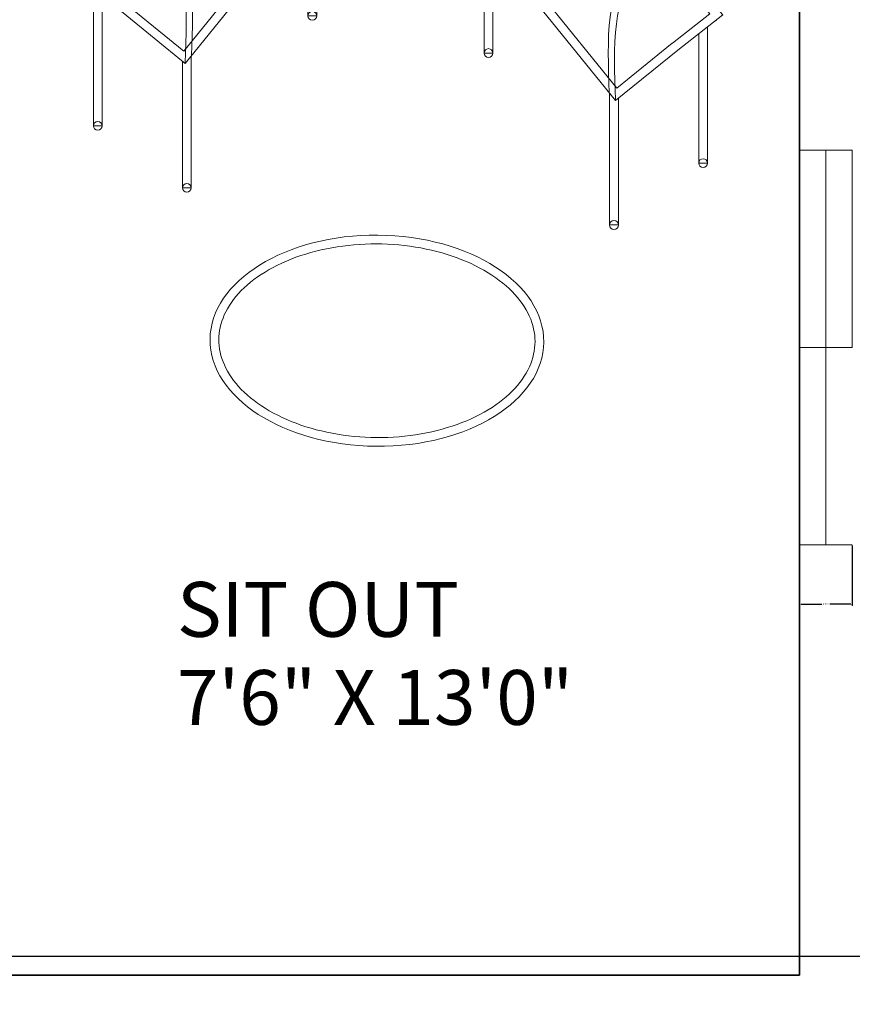
# Model space of a CAD drawing. Units: inches. Extents: x -61 to 1599, y -1316 to 257.
# Tile 192 of 204: x 1003 to 1098, y -173 to -61. Entities that reach past the tile are written whole.
import ezdxf

# ---------------------------------------------------------------- set-up
doc = ezdxf.new("R2010")
doc.units = ezdxf.units.IN
doc.header["$MEASUREMENT"] = 0
for name, color, linetype, lineweight in [('A-ANNO-DIMS', 2, 'Continuous', 18), ('A-AREA-IDEN', 1, 'Continuous', 18), ('FURNITURE', 83, 'Continuous', 18), ('WALLS', 4, 'Continuous', 35), ('WINDOWS', 220, 'Continuous', 18)]:
    doc.layers.add(name, color=color, linetype=linetype, lineweight=lineweight)
doc.styles.get("Standard").update_dxf_attribs({"font": 'arial.ttf'})
doc.dimstyles.get("Standard").update_dxf_attribs({"dimtxt": 0.18, "dimasz": 0.18, "dimexe": 0.18, "dimexo": 0.0625, "dimgap": 0.09, "dimtad": 0, "dimtih": 1, "dimtoh": 1, "dimdec": 0, "dimzin": 0, "dimdsep": 46, "dimlunit": 3, "dimtxsty": 'Standard', "dimcen": 0.09, "dimadec": 0, "dimazin": 0, "dimtfac": 1, "dimtdec": 0, "dimtofl": 0, "dimtmove": 0, "dimatfit": 3, "dimfxl": 1, "dimtolj": 1, "dimtzin": 0, "dimarcsym": 0})

# ---------------------------------------------------------------- blocks, each defined once
blk = doc.blocks.new('WIN-45IN')
for p, q in [((0, 44.83), (6, 44.83)), ((0, 0), (6, 0))]:
    blk.add_line(p, q)
for points in [[(6, 44.83), (3, 44.83), (3, 22.42), (6, 22.42)], [(3, 22.42), (0, 22.42), (0, 0), (3, 0)]]:
    blk.add_lwpolyline(points, close=True)
blk = doc.blocks.new('LOUNGE-CHAIR')
for p, q in [((14.76, 41.14), (14.76, 58.89)), ((14.04, 40.33), (14.04, 58.08)), ((6.52, 39.78), (9.29, 46.65)), ((6.58, 41.68), (8.18, 45.54)), ((7.84, 40.87), (9.45, 44.74)), ((1.64, 26.22), (1.64, 43.97)), ((0, 24.35), (16.38, 42.98)), ((0.97, 25.45), (0.97, 43.2)), ((0.97, 25.45), (0.97, 43.2)), ((16.38, 42.98), (20.51, 39.74)), ((16.97, 42.52), (16.97, 42.52)), ((1.45, 24.49), (16.5, 41.61)), ((16.5, 41.61), (19.89, 38.96)), ((15.97, 27.05), (15.97, 41.01)), ((16.97, 27.05), (16.97, 41.25)), ((20.51, 39.74), (27.76, 33.87)), ((19.88, 38.97), (26.35, 33.72)), ((12.02, 16.03), (26.35, 33.72)), ((12.16, 14.63), (27.76, 33.87)), ((27.1, 20.02), (27.1, 33.05)), ((26.1, 20.02), (26.1, 31.82)), ((16.97, 27.05), (15.97, 27.05)), ((0, 24.35), (5.1, 20.35)), ((0.75, 23.69), (0.79, 23.74)), ((1.45, 24.49), (5.72, 21.14)), ((1.73, 7.53), (1.73, 23)), ((2.73, 7.53), (2.73, 22.21)), ((5.1, 20.35), (12.16, 14.63)), ((5.73, 21.13), (12.02, 16.03)), ((27.1, 20.02), (26.1, 20.02)), ((11.85, 0.5), (11.85, 14.88)), ((12.85, 0.5), (12.85, 15.48)), ((2.73, 7.53), (1.73, 7.53)), ((12.85, 0.5), (11.85, 0.5))]:
    blk.add_line(p, q)
for centre in [(16.47, 27.05), (26.6, 20.02), (2.23, 7.53), (12.35, 0.5)]:
    blk.add_circle(centre, 0.5)
for centre, radius, start, end in [((23.93, 36.92), 23.8, 112.6586, 164.6996), ((30.25, 31.33), 31.28, 121.203, 156.1552)]:
    blk.add_arc(centre, radius, start, end)
for points, knots in [([(14.76, 49.49), (18.73, 49.7), (28.38, 50.23), (27.99, 39.93), (27.76, 33.87)], [0, 0, 0, 0, 10.281855, 24.983674, 24.983674, 24.983674, 24.983674]), ([(14.76, 48.72), (18.48, 48.91), (27.65, 49.16), (27.27, 39.12), (27.05, 33.06), (27.04, 33.03), (27.04, 33.01), (27.04, 32.98)], [0.614676, 0.614676, 0.614676, 0.614676, 10.281855, 24.983674, 24.983674, 24.983674, 25.041855, 25.041855, 25.041855, 25.041855]), ([(1.64, 31.22), (4.99, 31.37), (13.47, 31.24), (13.11, 21.57), (12.88, 15.51)], [1.527723, 1.527723, 1.527723, 1.527723, 10.281855, 24.983674, 24.983674, 24.983674, 24.983674]), ([(1.64, 30.44), (4.72, 30.55), (12.75, 30.17), (12.39, 20.76), (12.17, 14.7), (12.16, 14.67), (12.16, 14.65), (12.16, 14.63)], [2.150702, 2.150702, 2.150702, 2.150702, 10.281855, 24.983674, 24.983674, 24.983674, 25.041855, 25.041855, 25.041855, 25.041855])]:
    blk.add_open_spline(points, degree=3, knots=knots)
blk = doc.blocks.new('SIDE-TABLE-OVAL')
blk.add_ellipse((18.95, 11.99), major_axis=(-18.95, 0.16), ratio=0.632617)
blk.add_open_spline([(1, 12.14), (0.99, 11.17), (1.2, 10.2), (2.05, 8.28), (2.69, 7.34), (4.41, 5.58), (5.48, 4.76), (7.96, 3.32), (9.37, 2.71), (12.41, 1.74), (14.05, 1.4), (17.41, 1), (19.13, 0.95), (22.53, 1.15), (24.2, 1.41), (27.36, 2.19), (28.84, 2.73), (31.49, 4.02), (32.66, 4.78), (34.59, 6.45), (35.35, 7.36), (36.44, 9.24), (36.76, 10.2), (36.97, 12.14), (36.87, 13.11), (36.22, 15.04), (35.67, 16), (34.15, 17.81), (33.17, 18.67), (30.85, 20.19), (29.51, 20.86), (26.58, 21.94), (24.98, 22.36), (21.67, 22.89), (19.95, 23.01), (16.54, 22.94), (14.84, 22.76), (11.61, 22.1), (10.07, 21.63), (7.28, 20.44), (6.03, 19.73), (3.92, 18.13), (3.06, 17.25), (1.78, 15.4), (1.35, 14.44), (1.05, 13.03), (1, 12.59), (1, 12.14)], degree=3, knots=[0, 0, 0, 0, 0.279765, 0.279765, 0.559529, 0.559529, 0.839294, 0.839294, 1.119059, 1.119059, 1.398823, 1.398823, 1.678588, 1.678588, 1.958353, 1.958353, 2.238118, 2.238118, 2.517882, 2.517882, 2.797647, 2.797647, 3.077412, 3.077412, 3.357176, 3.357176, 3.636941, 3.636941, 3.916706, 3.916706, 4.19647, 4.19647, 4.476235, 4.476235, 4.756, 4.756, 5.035764, 5.035764, 5.315529, 5.315529, 5.595294, 5.595294, 5.875058, 5.875058, 6.154823, 6.154823, 6.283185, 6.283185, 6.283185, 6.283185])
blk = doc.blocks.new('*D647')
at = {"layer": 'A-ANNO-DIMS', "color": 0, "lineweight": -2, "transparency": 16777216}
for p, q in [((1091.7, -120.56), (1091.7, -127.4)), ((1097.7, -120.56), (1097.7, -127.4)), ((1091.88, -127.22), (1094.24, -127.22)), ((1097.52, -127.22), (1095.16, -127.22))]:
    blk.add_line(p, q, dxfattribs=at)
at = {"layer": 'A-ANNO-DIMS', "color": 0, "transparency": 16777216}
for points in [[(1091.88, -127.19), (1091.88, -127.25), (1091.7, -127.22)], [(1097.52, -127.19), (1097.52, -127.25), (1097.7, -127.22)]]:
    blk.add_solid(points, dxfattribs=at)
at = {"layer": 'DEFPOINTS', "color": 0, "transparency": 16777216}
for p in [(1091.7, -120.5), (1097.7, -120.5), (1097.7, -127.22)]:
    blk.add_point(p, dxfattribs=at)
at = {"layer": 'A-ANNO-DIMS', "color": 0, "transparency": 16777216, "insert": (1094.7, -127.22), "char_height": 0.18, "attachment_point": 5}
blk.add_mtext('\\A1;6 TYP.', dxfattribs=at)
blk = doc.blocks.new('*D698')
at = {"layer": 'A-ANNO-DIMS', "color": 0, "lineweight": -2, "transparency": 16777216}
for p, q in [((644.77, -167.17), (1598.48, -167.17)), ((1598.3, -167.35), (1598.3, -363.99)), ((1598.3, -560.99), (1598.3, -364.35)), ((644.77, -561.17), (1598.48, -561.17))]:
    blk.add_line(p, q, dxfattribs=at)
at = {"layer": 'A-ANNO-DIMS', "color": 0, "transparency": 16777216}
for points in [[(1598.27, -167.35), (1598.33, -167.35), (1598.3, -167.17)], [(1598.27, -560.99), (1598.33, -560.99), (1598.3, -561.17)]]:
    blk.add_solid(points, dxfattribs=at)
at = {"layer": 'DEFPOINTS', "color": 0, "transparency": 16777216}
for p in [(644.7, -167.17), (1598.3, -167.17), (644.7, -561.17)]:
    blk.add_point(p, dxfattribs=at)
at = {"layer": 'A-ANNO-DIMS', "color": 0, "transparency": 16777216, "insert": (1598.3, -364.17), "char_height": 0.18, "attachment_point": 5}
blk.add_mtext('\\A1;394', dxfattribs=at)

msp = doc.modelspace()

# ---------------------------------------------------------------- linework, layer by layer
at = {"layer": 'WALLS'}
for p, q in [((1091.7028, -169.3229), (1091.7028, -13.3229)), ((1001.7028, -169.3229), (1091.7028, -169.3229))]:
    msp.add_line(p, q, dxfattribs=at)

# ---------------------------------------------------------------- block references
at = {"layer": 'FURNITURE'}
for name, p in [('LOUNGE-CHAIR', (1009.776, -80.445)), ('SIDE-TABLE-OVAL', (1024.761, -109.297))]:
    msp.add_blockref(name, p, dxfattribs=at)
at = {"layer": 'FURNITURE', "extrusion": (0, 0, -1), "zscale": -1}
msp.add_blockref('LOUNGE-CHAIR', (-1082.9843, -84.6679), dxfattribs=at)
at = {"layer": 'WINDOWS'}
msp.add_blockref('WIN-45IN', (1091.703, -120.498), dxfattribs=at)

# ---------------------------------------------------------------- texts
at = {"layer": 'A-AREA-IDEN'}
for s, height, p in [('SIT OUT', 6.22364, (1021.0043, -130.923)), ('7\'6" X 13\'0"', 6.223643, (1021.0043, -140.9207))]:
    msp.add_text(s, height=height, dxfattribs=at).set_placement(p)

# ---------------------------------------------------------------- dimensions: what is measured, and where the dimension line sits
at = {"layer": 'A-ANNO-DIMS'}
dim = msp.add_linear_dim(base=(1097.7028, -127.2219), p1=(1091.7028, -120.4975), p2=(1097.7028, -120.4975), text='<> TYP.', dimstyle='Standard', override={"dimdec": 0, "dimlfac": 1, "dimrnd": 0, "dimzin": 0, "dimdsep": 46, "dimlunit": 2}, dxfattribs=at)
dim.commit()
dim.dimension.update_dxf_attribs({"geometry": '*D647', "text_midpoint": (1094.7028, -127.2219)})
dim = msp.add_linear_dim(base=(1598.3028, -167.169), p1=(644.7028, -561.169), p2=(644.7028, -167.169), angle=90, dimstyle='Standard', override={"dimdec": 0, "dimlfac": 1, "dimrnd": 0, "dimzin": 0, "dimdsep": 46, "dimlunit": 2}, dxfattribs=at)
dim.commit()
dim.dimension.update_dxf_attribs({"geometry": '*D698', "text_midpoint": (1598.3028, -364.169)})

doc.saveas('drawing.dxf')
